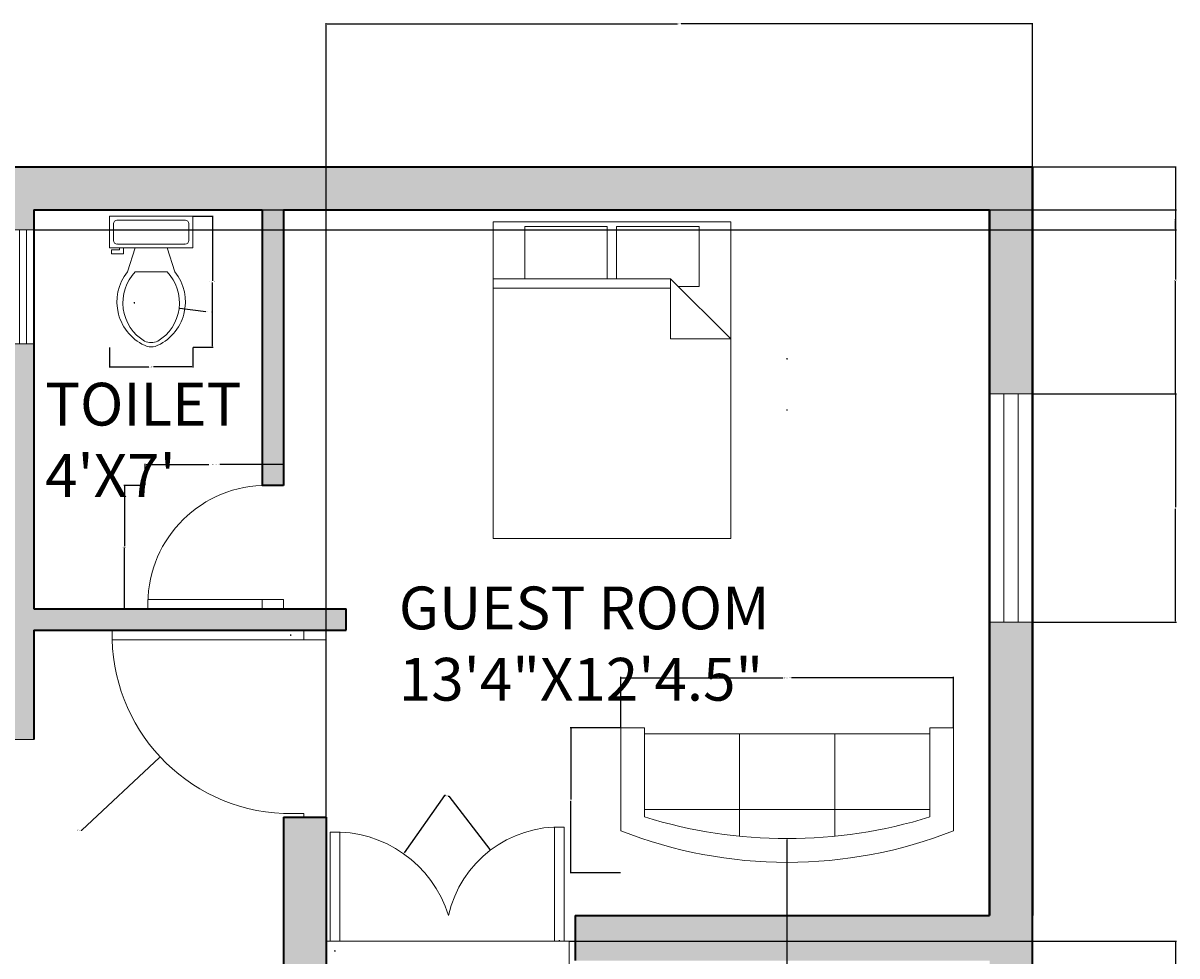
# Model space of a CAD drawing. Units: feet. Extents: x 1699 to 2359, y 1819 to 2211.
# Tile 4 of 4: x 2117 to 2359, y 2014 to 2211. Entities that reach past the tile are written whole.
import ezdxf

# ---------------------------------------------------------------- set-up
doc = ezdxf.new("R2010")
doc.units = ezdxf.units.FT
for name, color, linetype, lineweight in [('A-ANNO-DIMS', 2, 'Continuous', 18), ('A-AREA-IDEN', 7, 'Continuous', 18), ('A-DOOR', 4, 'Continuous', 18), ('A-FLOR', 7, 'Continuous', 18), ('A-FLOR-FIXT', 9, 'Continuous', 18), ('A-FURN', 8, 'Continuous', 18), ('A-GLAZ', 3, 'Continuous', 18), ('A-WALL', 7, 'Continuous', 35), ('A-WALL-PATT', 1, 'Continuous', 13)]:
    doc.layers.add(name, color=color, linetype=linetype, lineweight=lineweight)
doc.styles.get("Standard").update_dxf_attribs({"font": 'arial.ttf'})
doc.dimstyles.get("Standard").update_dxf_attribs({"dimtxt": 0.18, "dimasz": 0.18, "dimexe": 0.18, "dimexo": 0.0625, "dimgap": 0.09, "dimtad": 0, "dimtih": 1, "dimtoh": 1, "dimdec": 4, "dimzin": 0, "dimdsep": 46, "dimtxsty": 'Standard', "dimcen": 0.09, "dimadec": 0, "dimazin": 0, "dimtfac": 1, "dimtdec": 4, "dimtofl": 0, "dimtmove": 0, "dimatfit": 3, "dimfxl": 1, "dimtolj": 1, "dimtzin": 0, "dimarcsym": 0})

# ---------------------------------------------------------------- blocks, each defined once
blk = doc.blocks.new('Toilet - top')
for p, q in [((9.5, -6), (9.5, -2)), ((-10, -8.5), (-8, -8.5)), ((-10, -9.5), (-10, -8.5)), ((-8, -8.5), (-8, -8)), ((-7, -8), (-7, -9.5)), ((-4, -8), (-6, -14)), ((4, -8), (6, -14)), ((-7, -9.5), (-10, -9.5)), ((4, -14), (-4, -14))]:
    blk.add_line(p, q)
blk.add_lwpolyline([(10.5, -8), (10.5, 0), (-10.5, 0), (-10.5, -8)], close=True)
for points in [[(-9.5, -2), (-9.5, -6)], [(8.5, -1), (-8.5, -1)], [(-8.5, -7), (8.5, -7)]]:
    blk.add_lwpolyline(points)
for centre, radius, start, end in [((-8.62, -1.88), 0.884, 81.8699, 188.1301), ((8.62, -1.88), 0.884, 351.8699, 98.1301), ((-8.62, -6.12), 0.884, 171.8699, 278.1301), ((8.62, -6.12), 0.884, 261.8699, 8.1301), ((3.52, -21.58), 12.17, 141.4691, 247.9714), ((4.2, -21.82), 11.33, 136.3677, 238.9468), ((-3.52, -21.58), 12.17, 292.0284, 38.5307), ((-4.2, -21.82), 11.33, 301.053, 43.6321), ((0, -27.88), 4, 245.7318, 294.2682), ((0, -29), 4, 254.8605, 285.1395)]:
    blk.add_arc(centre, radius, start, end)
blk = doc.blocks.new('Bed - Queen')
for p, q in [((0, -80.00003), (0, 0)), ((0, 0), (59.99999, 0)), ((59.99999, 0), (59.99999, -80.00003)), ((7.99999, -1.2), (28.79998, -1.2)), ((7.99999, -14.4), (7.99999, -1.2)), ((28.79998, -1.2), (28.79998, -14.4)), ((31.19999, -1.2), (51.99999, -1.2)), ((31.19999, -14.4), (31.19999, -1.2)), ((51.99999, -1.2), (51.99999, -16.4)), ((0, -14.4), (44.8, -14.4)), ((59.99999, -29.6), (44.8, -14.4)), ((44.8, -14.4), (44.8, -29.6)), ((44.8, -16.8), (0, -16.8)), ((51.99999, -16.4), (46.79936, -16.4)), ((44.8, -29.6), (59.99999, -29.6)), ((59.99999, -80.00003), (0, -80.00003))]:
    blk.add_line(p, q)
blk = doc.blocks.new('Sofa - Roundback 7 ft.')
for p, q in [((-12.00002, -32.4421), (-12.00003, -6.5971)), ((11.99997, -32.4421), (11.99998, -6.5971)), ((-36.000027, -34), (-36.000027, -11.4696)), ((35.99998, -34), (35.99998, -11.4696)), ((-35.999844, -13.3819), (35.9998, -13.3819)), ((-36.000027, -32.4421), (35.99998, -32.4421))]:
    blk.add_line(p, q)
for points in [[(-36.000027, -34), (-42.000027, -34), (-42.000027, -8)], [(41.99998, -8), (41.99998, -34), (35.99998, -34)]]:
    blk.add_lwpolyline(points)
for centre, radius, start, end in [((0, -114.25), 114.25, 68.43141, 111.5686), ((-0.00001, -127.1968), 121.1968, 72.72033, 107.2797)]:
    blk.add_arc(centre, radius, start, end)
blk = doc.blocks.new('WIN-24-PARTITION')
for p, q in [((0, 24), (4.5, 24)), ((0, 0), (0, 24)), ((1.5, 0), (1.5, 24)), ((3, 0), (3, 24)), ((4.5, 24), (4.5, 0)), ((4.5, 0), (0, 0))]:
    blk.add_line(p, q)
blk = doc.blocks.new('DOOR-SWING-24')
for p, q in [((0.02, 0), (0.02, 2)), ((0.02, 2), (28.52, 2)), ((24.02, 0), (0.02, 0))]:
    blk.add_line(p, q)
blk.add_arc((25.02, 1), 25.02, 92.2906, 182.2906)
blk = doc.blocks.new('*D12')
at = {"layer": 'A-ANNO-DIMS', "color": 0, "lineweight": -2, "transparency": 16777216}
for p, q in [((2242.38, 2062.41), (2242.38, 2073.03)), ((2242.56, 2072.85), (2276.47, 2072.85)), ((2312.2, 2072.85), (2278.28, 2072.85)), ((2312.38, 2062.41), (2312.38, 2073.03))]:
    blk.add_line(p, q, dxfattribs=at)
at = {"layer": 'A-ANNO-DIMS', "color": 0, "transparency": 16777216}
for points in [[(2242.56, 2072.88), (2242.56, 2072.82), (2242.38, 2072.85)], [(2312.2, 2072.88), (2312.2, 2072.82), (2312.38, 2072.85)]]:
    blk.add_solid(points, dxfattribs=at)
at = {"layer": 'Defpoints', "color": 0, "transparency": 16777216}
for p in [(2242.38, 2072.85), (2242.38, 2062.35), (2312.38, 2062.35)]:
    blk.add_point(p, dxfattribs=at)
at = {"layer": 'A-ANNO-DIMS', "color": 0, "transparency": 16777216, "insert": (2277.38, 2072.85), "char_height": 0.18, "attachment_point": 5}
blk.add_mtext('\\A1;SOFA 70 TYP.', dxfattribs=at)
blk = doc.blocks.new('*D13')
at = {"layer": 'A-ANNO-DIMS', "color": 0, "lineweight": -2, "transparency": 16777216}
for p, q in [((2242.31, 2062.35), (2231.7, 2062.35)), ((2231.88, 2062.17), (2231.88, 2047.25)), ((2231.88, 2031.97), (2231.88, 2046.89)), ((2242.31, 2031.79), (2231.7, 2031.79))]:
    blk.add_line(p, q, dxfattribs=at)
at = {"layer": 'A-ANNO-DIMS', "color": 0, "transparency": 16777216}
for points in [[(2231.85, 2062.17), (2231.91, 2062.17), (2231.88, 2062.35)], [(2231.85, 2031.97), (2231.91, 2031.97), (2231.88, 2031.79)]]:
    blk.add_solid(points, dxfattribs=at)
at = {"layer": 'Defpoints', "color": 0, "transparency": 16777216}
for p in [(2242.38, 2062.35), (2231.88, 2031.79), (2242.38, 2031.79)]:
    blk.add_point(p, dxfattribs=at)
at = {"layer": 'A-ANNO-DIMS', "color": 0, "transparency": 16777216, "insert": (2231.88, 2047.07), "char_height": 0.18, "attachment_point": 5}
blk.add_mtext('\\A1;31 TYP.', dxfattribs=at)
blk = doc.blocks.new('*D14')
at = {"layer": 'A-ANNO-DIMS', "color": 0, "lineweight": -2, "transparency": 16777216}
for p, q in [((2152.43, 2169.97), (2156.68, 2169.97)), ((2156.5, 2169.79), (2156.5, 2156.38)), ((2156.5, 2142.61), (2156.5, 2156.02)), ((2152.43, 2142.43), (2156.68, 2142.43))]:
    blk.add_line(p, q, dxfattribs=at)
at = {"layer": 'A-ANNO-DIMS', "color": 0, "transparency": 16777216}
for points in [[(2156.47, 2169.79), (2156.53, 2169.79), (2156.5, 2169.97)], [(2156.47, 2142.61), (2156.53, 2142.61), (2156.5, 2142.43)]]:
    blk.add_solid(points, dxfattribs=at)
at = {"layer": 'Defpoints', "color": 0, "transparency": 16777216}
for p in [(2152.37, 2169.97), (2156.5, 2169.97), (2152.37, 2142.43)]:
    blk.add_point(p, dxfattribs=at)
at = {"layer": 'A-ANNO-DIMS', "color": 0, "transparency": 16777216, "insert": (2156.5, 2156.2), "char_height": 0.18, "attachment_point": 5}
blk.add_mtext('\\A1;WC 28 TYP.', dxfattribs=at)
blk = doc.blocks.new('*D15')
at = {"layer": 'A-ANNO-DIMS', "color": 0, "lineweight": -2, "transparency": 16777216}
for p, q in [((2134.87, 2142.37), (2134.87, 2138.12)), ((2152.37, 2142.37), (2152.37, 2138.12)), ((2135.05, 2138.3), (2143.1, 2138.3)), ((2152.19, 2138.3), (2144.13, 2138.3))]:
    blk.add_line(p, q, dxfattribs=at)
at = {"layer": 'A-ANNO-DIMS', "color": 0, "transparency": 16777216}
for points in [[(2135.05, 2138.33), (2135.05, 2138.27), (2134.87, 2138.3)], [(2152.19, 2138.33), (2152.19, 2138.27), (2152.37, 2138.3)]]:
    blk.add_solid(points, dxfattribs=at)
at = {"layer": 'Defpoints', "color": 0, "transparency": 16777216}
for p in [(2134.87, 2142.43), (2152.37, 2142.43), (2152.37, 2138.3)]:
    blk.add_point(p, dxfattribs=at)
at = {"layer": 'A-ANNO-DIMS', "color": 0, "transparency": 16777216, "insert": (2143.62, 2138.3), "char_height": 0.18, "attachment_point": 5}
blk.add_mtext('\\A1;18 TYP.', dxfattribs=at)
blk = doc.blocks.new('*D18')
at = {"layer": 'A-ANNO-DIMS', "color": 0, "lineweight": -2, "transparency": 16777216}
for p, q in [((2142.37, 2113.41), (2142.37, 2117.89)), ((2142.55, 2117.71), (2155.77, 2117.71)), ((2171.25, 2117.71), (2158.03, 2117.71)), ((2171.43, 2113.41), (2171.43, 2117.89))]:
    blk.add_line(p, q, dxfattribs=at)
at = {"layer": 'A-ANNO-DIMS', "color": 0, "transparency": 16777216}
for points in [[(2142.55, 2117.74), (2142.55, 2117.68), (2142.37, 2117.71)], [(2171.25, 2117.74), (2171.25, 2117.68), (2171.43, 2117.71)]]:
    blk.add_solid(points, dxfattribs=at)
at = {"layer": 'Defpoints', "color": 0, "transparency": 16777216}
for p in [(2171.43, 2117.71), (2142.37, 2113.35), (2171.43, 2113.35)]:
    blk.add_point(p, dxfattribs=at)
at = {"layer": 'A-ANNO-DIMS', "color": 0, "transparency": 16777216, "insert": (2156.9, 2117.71), "char_height": 0.18, "attachment_point": 5}
blk.add_mtext('\\A1;DOOR D1 29 TYP.', dxfattribs=at)
blk = doc.blocks.new('*D19')
at = {"layer": 'A-ANNO-DIMS', "color": 0, "lineweight": -2, "transparency": 16777216}
for p, q in [((2142.31, 2113.35), (2137.84, 2113.35)), ((2138.02, 2113.17), (2138.02, 2100.53)), ((2138.02, 2087.53), (2138.02, 2100.17)), ((2142.31, 2087.35), (2137.84, 2087.35))]:
    blk.add_line(p, q, dxfattribs=at)
at = {"layer": 'A-ANNO-DIMS', "color": 0, "transparency": 16777216}
for points in [[(2137.99, 2113.17), (2138.05, 2113.17), (2138.02, 2113.35)], [(2137.99, 2087.53), (2138.05, 2087.53), (2138.02, 2087.35)]]:
    blk.add_solid(points, dxfattribs=at)
at = {"layer": 'Defpoints', "color": 0, "transparency": 16777216}
for p in [(2138.02, 2113.35), (2142.37, 2113.35), (2142.37, 2087.35)]:
    blk.add_point(p, dxfattribs=at)
at = {"layer": 'A-ANNO-DIMS', "color": 0, "transparency": 16777216, "insert": (2138.02, 2100.35), "char_height": 0.18, "attachment_point": 5}
blk.add_mtext('\\A1;26 TYP.', dxfattribs=at)
blk = doc.blocks.new('*D22')
at = {"layer": 'A-ANNO-DIMS', "color": 0, "lineweight": -2, "transparency": 16777216}
for p, q in [((2180.43, 1853.41), (2180.43, 2210.63)), ((2328.93, 1848.91), (2328.93, 2210.63)), ((2180.61, 2210.45), (2254.29, 2210.45)), ((2328.75, 2210.45), (2255.06, 2210.45))]:
    blk.add_line(p, q, dxfattribs=at)
at = {"layer": 'A-ANNO-DIMS', "color": 0, "transparency": 16777216}
for points in [[(2180.61, 2210.48), (2180.61, 2210.42), (2180.43, 2210.45)], [(2328.75, 2210.48), (2328.75, 2210.42), (2328.93, 2210.45)]]:
    blk.add_solid(points, dxfattribs=at)
at = {"layer": 'Defpoints', "color": 0, "transparency": 16777216}
for p in [(2328.93, 2210.45), (2180.43, 1853.35), (2328.93, 1848.85)]:
    blk.add_point(p, dxfattribs=at)
at = {"layer": 'A-ANNO-DIMS', "color": 0, "transparency": 16777216, "insert": (2254.68, 2210.45), "char_height": 0.18, "attachment_point": 5}
blk.add_mtext('\\A1;148.5', dxfattribs=at)
blk = doc.blocks.new('*D35')
at = {"layer": 'A-ANNO-DIMS', "color": 0, "lineweight": -2, "transparency": 16777216}
for p, q in [((2231.55, 2017.45), (2359.21, 2017.45)), ((2359.03, 2017.27), (2359.03, 1976.45)), ((2359.03, 1935.26), (2359.03, 1976.08)), ((2231.55, 1935.08), (2359.21, 1935.08))]:
    blk.add_line(p, q, dxfattribs=at)
at = {"layer": 'A-ANNO-DIMS', "color": 0, "transparency": 16777216}
for points in [[(2359, 2017.27), (2359.06, 2017.27), (2359.03, 2017.45)], [(2359, 1935.26), (2359.06, 1935.26), (2359.03, 1935.08)]]:
    blk.add_solid(points, dxfattribs=at)
at = {"layer": 'Defpoints', "color": 0, "transparency": 16777216}
for p in [(2231.49, 2017.45), (2359.03, 2017.45), (2231.49, 1935.08)]:
    blk.add_point(p, dxfattribs=at)
at = {"layer": 'A-ANNO-DIMS', "color": 0, "transparency": 16777216, "insert": (2359.03, 1976.26), "char_height": 0.18, "attachment_point": 5}
blk.add_mtext('\\A1;82.37', dxfattribs=at)
blk = doc.blocks.new('*D36')
at = {"layer": 'A-ANNO-DIMS', "color": 0, "lineweight": -2, "transparency": 16777216}
for p, q in [((2328.99, 2132.58), (2359.21, 2132.58)), ((2359.03, 2132.4), (2359.03, 2108.76)), ((2359.03, 2084.76), (2359.03, 2108.4)), ((2328.99, 2084.58), (2359.21, 2084.58))]:
    blk.add_line(p, q, dxfattribs=at)
at = {"layer": 'A-ANNO-DIMS', "color": 0, "transparency": 16777216}
for points in [[(2359, 2132.4), (2359.06, 2132.4), (2359.03, 2132.58)], [(2359, 2084.76), (2359.06, 2084.76), (2359.03, 2084.58)]]:
    blk.add_solid(points, dxfattribs=at)
at = {"layer": 'Defpoints', "color": 0, "transparency": 16777216}
for p in [(2328.93, 2132.58), (2359.03, 2132.58), (2328.93, 2084.58)]:
    blk.add_point(p, dxfattribs=at)
at = {"layer": 'A-ANNO-DIMS', "color": 0, "transparency": 16777216, "insert": (2359.03, 2108.58), "char_height": 0.18, "attachment_point": 5}
blk.add_mtext('\\A1;48', dxfattribs=at)
blk = doc.blocks.new('*D37')
at = {"layer": 'A-ANNO-DIMS', "color": 0, "lineweight": -2, "transparency": 16777216}
for p, q in [((2328.989154, 2180.349391), (2359.206654, 2180.349391)), ((2359.026654, 2180.169391), (2359.026654, 2156.643959)), ((2359.026654, 2132.758527), (2359.026654, 2156.283959)), ((2328.989154, 2132.578527), (2359.206654, 2132.578527))]:
    blk.add_line(p, q, dxfattribs=at)
at = {"layer": 'A-ANNO-DIMS', "color": 0, "transparency": 16777216}
for points in [[(2358.996654, 2180.169391), (2359.056654, 2180.169391), (2359.026654, 2180.349391)], [(2358.996654, 2132.758527), (2359.056654, 2132.758527), (2359.026654, 2132.578527)]]:
    blk.add_solid(points, dxfattribs=at)
at = {"layer": 'Defpoints', "color": 0, "transparency": 16777216}
for p in [(2328.926654, 2180.349391), (2359.026654, 2180.349391), (2328.926654, 2132.578527)]:
    blk.add_point(p, dxfattribs=at)
at = {"layer": 'A-ANNO-DIMS', "color": 0, "transparency": 16777216, "insert": (2359.026654, 2156.463959), "char_height": 0.18, "attachment_point": 5}
blk.add_mtext('\\A1;47.77', dxfattribs=at)
blk = doc.blocks.new('*D51')
at = {"layer": 'A-ANNO-DIMS', "color": 0, "lineweight": -2, "transparency": 16777216}
for p, q in [((2118.99, 2171.35), (2359.21, 2171.35)), ((2359.03, 2171.17), (2359.03, 2169.43)), ((2118.99, 2167.14), (2359.21, 2167.14)), ((2359.03, 2167.32), (2359.03, 2169.06))]:
    blk.add_line(p, q, dxfattribs=at)
at = {"layer": 'A-ANNO-DIMS', "color": 0, "transparency": 16777216}
for points in [[(2359, 2171.17), (2359.06, 2171.17), (2359.03, 2171.35)], [(2359, 2167.32), (2359.06, 2167.32), (2359.03, 2167.14)]]:
    blk.add_solid(points, dxfattribs=at)
at = {"layer": 'Defpoints', "color": 0, "transparency": 16777216}
for p in [(2118.93, 2171.35), (2118.93, 2167.14), (2359.03, 2167.14)]:
    blk.add_point(p, dxfattribs=at)
at = {"layer": 'A-ANNO-DIMS', "color": 0, "transparency": 16777216, "insert": (2359.03, 2169.25), "char_height": 0.18, "attachment_point": 5}
blk.add_mtext('\\A1;4.21', dxfattribs=at)
blk = doc.blocks.new('*D55')
at = {"layer": 'A-ANNO-DIMS', "color": 0, "lineweight": -2, "transparency": 16777216}
for p, q in [((2172.91, 2081.85), (2173.09, 2081.85)), ((2173, 2081.76), (2173, 2081.94)), ((2129.04, 2040.8), (2145.4, 2056.07)), ((2128.86, 2040.8), (2129.04, 2040.8))]:
    blk.add_line(p, q, dxfattribs=at)
at = {"layer": 'A-ANNO-DIMS', "color": 0, "transparency": 16777216}
blk.add_solid([(2145.38, 2056.1), (2145.42, 2056.05), (2145.53, 2056.2)], dxfattribs=at)
at = {"layer": 'Defpoints', "color": 0, "transparency": 16777216}
for p in [(2173, 2081.85), (2145.53, 2056.2)]:
    blk.add_point(p, dxfattribs=at)
at = {"layer": 'A-ANNO-DIMS', "color": 0, "transparency": 16777216, "insert": (2128.38, 2040.8), "char_height": 0.18, "attachment_point": 5}
blk.add_mtext('\\A1;R37.59', dxfattribs=at)
blk = doc.blocks.new('*D57')
at = {"layer": 'A-ANNO-DIMS', "color": 0, "lineweight": -2, "transparency": 16777216}
for p, q in [((2205.33, 2048.11), (2196.79, 2035.99)), ((2205.51, 2048.11), (2205.33, 2048.11)), ((2182.18, 2015.4), (2182.36, 2015.4)), ((2182.27, 2015.31), (2182.27, 2015.49))]:
    blk.add_line(p, q, dxfattribs=at)
at = {"layer": 'A-ANNO-DIMS', "color": 0, "transparency": 16777216}
blk.add_solid([(2196.76, 2036), (2196.81, 2035.97), (2196.68, 2035.84)], dxfattribs=at)
at = {"layer": 'Defpoints', "color": 0, "transparency": 16777216}
for p in [(2196.68, 2035.84), (2182.27, 2015.4)]:
    blk.add_point(p, dxfattribs=at)
at = {"layer": 'A-ANNO-DIMS', "color": 0, "transparency": 16777216, "insert": (2205.98, 2048.11), "char_height": 0.18, "attachment_point": 5}
blk.add_mtext('\\A1;R25.01', dxfattribs=at)
blk = doc.blocks.new('*D58')
at = {"layer": 'A-ANNO-DIMS', "color": 0, "lineweight": -2, "transparency": 16777216}
for p, q in [((2206.04, 2047.94), (2206.22, 2047.94)), ((2206.22, 2047.94), (2214.82, 2036.7)), ((2229.37, 2017.57), (2229.55, 2017.57)), ((2229.46, 2017.48), (2229.46, 2017.66))]:
    blk.add_line(p, q, dxfattribs=at)
at = {"layer": 'A-ANNO-DIMS', "color": 0, "transparency": 16777216}
blk.add_solid([(2214.85, 2036.71), (2214.8, 2036.68), (2214.93, 2036.55)], dxfattribs=at)
at = {"layer": 'Defpoints', "color": 0, "transparency": 16777216}
for p in [(2214.93, 2036.55), (2229.46, 2017.57)]:
    blk.add_point(p, dxfattribs=at)
at = {"layer": 'A-ANNO-DIMS', "color": 0, "transparency": 16777216, "insert": (2205.49, 2047.94), "char_height": 0.18, "attachment_point": 5}
blk.add_mtext('\\A1;R23.903', dxfattribs=at)
blk = doc.blocks.new('*D59')
at = {"layer": 'A-ANNO-DIMS', "color": 0, "lineweight": -2, "transparency": 16777216}
for p, q in [((2277.29, 2140.01), (2277.47, 2140.01)), ((2277.38, 2139.92), (2277.38, 2140.1)), ((2277.38, 1978.42), (2277.38, 2038.84)), ((2277.56, 1978.42), (2277.38, 1978.42))]:
    blk.add_line(p, q, dxfattribs=at)
at = {"layer": 'A-ANNO-DIMS', "color": 0, "transparency": 16777216}
blk.add_solid([(2277.41, 2038.84), (2277.35, 2038.84), (2277.38, 2039.02)], dxfattribs=at)
at = {"layer": 'Defpoints', "color": 0, "transparency": 16777216}
for p in [(2277.38, 2140.01), (2277.38, 2039.02)]:
    blk.add_point(p, dxfattribs=at)
at = {"layer": 'A-ANNO-DIMS', "color": 0, "transparency": 16777216, "insert": (2278.11, 1978.42), "char_height": 0.18, "attachment_point": 5}
blk.add_mtext('\\A1;2X R101', dxfattribs=at)
blk = doc.blocks.new('*D60')
at = {"layer": 'A-ANNO-DIMS', "color": 0, "lineweight": -2, "transparency": 16777216}
for p, q in [((2277.29, 2129.22), (2277.47, 2129.22)), ((2277.38, 2129.13), (2277.38, 2129.31)), ((2277.38, 1976.89), (2277.38, 2033.84)), ((2277.56, 1976.89), (2277.38, 1976.89))]:
    blk.add_line(p, q, dxfattribs=at)
at = {"layer": 'A-ANNO-DIMS', "color": 0, "transparency": 16777216}
blk.add_solid([(2277.41, 2033.84), (2277.35, 2033.84), (2277.38, 2034.02)], dxfattribs=at)
at = {"layer": 'Defpoints', "color": 0, "transparency": 16777216}
for p in [(2277.38, 2129.22), (2277.38, 2034.02)]:
    blk.add_point(p, dxfattribs=at)
at = {"layer": 'A-ANNO-DIMS', "color": 0, "transparency": 16777216, "insert": (2278.16, 1976.89), "char_height": 0.18, "attachment_point": 5}
blk.add_mtext('\\A1;2X R95.2', dxfattribs=at)
blk = doc.blocks.new('*D64')
at = {"layer": 'A-ANNO-DIMS', "color": 0, "lineweight": -2, "transparency": 16777216}
for p, q in [((2140.03, 2151.79), (2140.21, 2151.79)), ((2140.12, 2151.7), (2140.12, 2151.88)), ((2155.09, 2149.84), (2149.66, 2150.54))]:
    blk.add_line(p, q, dxfattribs=at)
at = {"layer": 'A-ANNO-DIMS', "color": 0, "transparency": 16777216}
blk.add_solid([(2149.66, 2150.57), (2149.65, 2150.52), (2149.48, 2150.57)], dxfattribs=at)
at = {"layer": 'Defpoints', "color": 0, "transparency": 16777216}
for p in [(2140.12, 2151.79), (2149.48, 2150.57)]:
    blk.add_point(p, dxfattribs=at)
at = {"layer": 'A-ANNO-DIMS', "color": 0, "transparency": 16777216, "insert": (2155.75, 2149.84), "char_height": 0.18, "attachment_point": 5}
blk.add_mtext('\\A1;4X R9.441', dxfattribs=at)

msp = doc.modelspace()

# ---------------------------------------------------------------- hatches: boundary and pattern name
at = {"layer": 'A-WALL-PATT'}
h = msp.add_hatch(color=256, dxfattribs=at)
h.dxf.hatch_style = 1
h.paths.add_polyline_path([(2180.4267, 1853.3494), (2180.4267, 1857.8494), (1955.4267, 1857.8494), (1955.4267, 1935.0782), (1991.4267, 1935.0782), (1991.4267, 1939.5782), (1955.4267, 1939.5782), (1955.4267, 2022.8494), (1950.9267, 2022.8494), (1950.9267, 1857.8494), (1784.4267, 1857.8494), (1784.4267, 1908.7829), (1775.4267, 1908.7829), (1775.4267, 1853.3494), (1733.9267, 1853.3494), (1733.9267, 2018.3494), (1775.4267, 2018.3494), (1775.4267, 2022.8494), (1738.4267, 2022.8494), (1738.4267, 2171.3494), (1898.4267, 2171.3494), (1898.4267, 2060.8494), (1902.9267, 2060.8494), (1902.9267, 2064.8494), (1955.4267, 2064.8494), (1955.4267, 2069.3494), (1902.9267, 2069.3494), (1902.9267, 2171.3494), (1950.9267, 2171.3494), (1950.9267, 2169.0373), (1955.4267, 2169.0373), (1955.4267, 2175.8494), (2114.4267, 2175.8494), (2114.4267, 2167.1408), (2118.9267, 2167.1408), (2118.9267, 2171.3494), (2166.9267, 2171.3494), (2166.9267, 2113.3494), (2171.4267, 2113.3494), (2171.4267, 2171.3494), (2319.9267, 2171.3494), (2319.9267, 2132.5785), (2328.9267, 2132.5785), (2328.9267, 2180.3494), (2309.4267, 2180.3494), (1729.4267, 2180.3494), (1729.4267, 1848.8494), (2180.4267, 1848.8494)])
h.paths.add_polyline_path([(1784.4267, 1987.6139), (1775.4267, 1987.6139), (1775.4267, 1944.7829), (1784.4267, 1944.7829)], flags=17)
h.paths.add_polyline_path([(1912.9267, 2022.8494), (1775.4267, 2022.8494), (1775.4267, 2013.6139), (1784.4267, 2013.6139), (1784.4267, 2018.3494), (1912.9267, 2018.3494)], flags=17)
h.paths.add_polyline_path([(2018.4267, 2135.3494), (2047.4307, 2135.3494), (2047.4307, 2139.8494), (1981.4267, 2139.8494), (1981.4267, 2135.3494), (2013.9267, 2135.3494), (2013.9267, 2059.8494), (2018.4267, 2059.8494)], flags=17)
h.paths.add_polyline_path([(2114.4267, 2139.8494), (2071.4307, 2139.8494), (2071.4307, 2135.3494), (2114.4267, 2135.3494)], flags=17)
h.paths.add_polyline_path([(2118.9267, 2143.1408), (2114.4267, 2143.1408), (2114.4267, 2059.8494), (2118.9267, 2059.8494), (2118.9267, 2082.8494), (2184.631, 2082.8494), (2184.631, 2087.3494), (2118.9267, 2087.3494)], flags=17)
h.paths.add_polyline_path([(2328.9267, 2084.5785), (2319.9267, 2084.5785), (2319.9267, 2022.8494), (2232.7955, 2022.8494), (2232.7955, 2013.3494), (2319.9267, 2013.3494), (2319.9267, 1998.3723), (2328.9267, 1998.3723)], flags=17)
h.paths.add_polyline_path([(2180.4267, 2043.5261), (2171.4267, 2043.5261), (2171.4267, 2006.4114), (2180.4267, 2006.4114)], flags=17)
h.paths.add_polyline_path([(2015.0526, 1939.5782), (1991.4267, 1939.5782), (1991.4267, 1935.0782), (2015.0526, 1935.0782)], flags=17)
h.paths.add_polyline_path([(2180.4267, 1939.5782), (2087.0526, 1939.5782), (2087.0526, 1935.0782), (2180.4267, 1935.0782)], flags=17)
h.paths.add_polyline_path([(2328.9267, 1868.1839), (2319.9267, 1868.1839), (2319.9267, 1853.3494), (2180.4267, 1853.3494), (2180.4267, 1848.8494), (2328.9267, 1848.8494)], flags=17)

# ---------------------------------------------------------------- linework, layer by layer
at = {"layer": 'A-DOOR'}
for p, q in [((2166.9267, 2089.3494), (2166.9267, 2087.3494)), ((2171.4267, 2089.3494), (2171.4267, 2087.3494)), ((2171.4267, 2082.8494), (2135.4267, 2082.8494)), ((2135.4267, 2082.8494), (2135.4267, 2080.8494)), ((2175.7191, 2082.7861), (2175.7191, 2080.8494)), ((2180.4267, 2082.8494), (2180.4267, 2080.8494)), ((2135.4267, 2080.8494), (2180.4267, 2080.8494)), ((2175.7191, 2044.2932), (2171.4267, 2044.2932)), ((2175.7191, 2044.2932), (2175.7191, 2043.5261)), ((2230.4592, 2041.4514), (2228.4592, 2041.4514)), ((2228.4592, 2041.4514), (2228.4592, 2017.4514)), ((2230.4592, 2017.4514), (2230.4592, 2041.4514)), ((2181.2703, 2022.8494), (2181.2703, 2040.3914)), ((2181.2703, 2040.3914), (2183.2703, 2040.3914)), ((2183.2703, 2040.3914), (2183.2703, 2017.4514)), ((2181.2703, 2022.8494), (2181.2703, 2017.4514)), ((2180.4267, 2017.4514), (2182.4016, 2017.4514)), ((2228.4592, 2017.4514), (2180.4267, 2017.4514)), ((2182.4592, 2017.4514), (2183.2703, 2017.4514)), ((2228.4592, 2017.4514), (2230.4592, 2017.4514)), ((2230.4592, 2017.4514), (2232.7955, 2017.4514))]:
    msp.add_line(p, q, dxfattribs=at)
for centre, radius, start, end in [((2173.0026, 2081.8494), 37.5892, 178.475559, 267.597193), ((2229.4592, 2017.5698), 23.9025, 87.602239, 167.239361), ((2182.2703, 2015.3995), 25.012, 17.328754, 92.291346)]:
    msp.add_arc(centre, radius, start, end, dxfattribs=at)
at = {"layer": 'A-FLOR'}
for p, q in [((2013.9267, 2059.8494), (2118.9267, 2059.8494)), ((2231.4915, 1935.0782), (2231.4915, 2017.4514))]:
    msp.add_line(p, q, dxfattribs=at)
at = {"layer": 'A-GLAZ'}
for p, q in [((2328.9267, 2132.5785), (2319.9267, 2132.5785)), ((2319.9267, 2132.5785), (2319.9267, 2084.5785)), ((2322.9267, 2132.5785), (2322.9267, 2084.5785)), ((2325.9267, 2132.5785), (2325.9267, 2084.5785)), ((2328.9267, 2084.5785), (2328.9267, 2132.5785)), ((2319.9267, 2084.5785), (2328.9267, 2084.5785))]:
    msp.add_line(p, q, dxfattribs=at)
at = {"layer": 'A-WALL'}
for p, q in [((1729.4267, 2180.3494), (2309.4267, 2180.3494)), ((2309.4267, 2180.3494), (2328.9267, 2180.3494)), ((2328.9267, 2180.3494), (2328.9267, 2022.8494)), ((2328.9267, 1998.3723), (2328.9267, 2180.2967)), ((2118.9267, 2171.3494), (2118.9267, 2087.3494)), ((2118.9267, 2171.3494), (2166.9267, 2171.3494)), ((2166.9267, 2171.3494), (2166.9267, 2113.3494)), ((2171.4267, 2171.3494), (2171.4267, 2113.3494)), ((2171.4267, 2171.3494), (2319.9267, 2171.3494)), ((2319.9267, 2171.3494), (2319.9267, 2022.8494)), ((2319.9267, 2022.8494), (2319.9267, 2171.3494)), ((2171.4267, 2113.3494), (2166.9267, 2113.3494)), ((2118.9267, 2087.3494), (2184.631, 2087.3494)), ((2184.631, 2082.8494), (2184.631, 2087.3494)), ((2118.9267, 2082.8494), (2184.631, 2082.8494)), ((2118.9267, 2082.8494), (2118.9267, 2059.8494)), ((2171.4267, 2043.5261), (2180.4267, 2043.5261)), ((2171.4267, 2043.5261), (2171.4267, 2006.4114)), ((2180.4267, 2043.5261), (2180.4267, 2006.4114)), ((2232.7955, 2022.8494), (2319.9267, 2022.8494)), ((2232.7955, 2022.8494), (2232.7955, 2013.3494))]:
    msp.add_line(p, q, dxfattribs=at)

# ---------------------------------------------------------------- block references
at = {"layer": 'A-DOOR'}
msp.add_blockref('DOOR-SWING-24', (2142.908, 2087.349), dxfattribs=at)
at = {"layer": 'A-FLOR-FIXT', "xscale": 0.8333333333333331, "yscale": 0.8333333333333331, "zscale": 0.8333333333333331}
msp.add_blockref('Toilet - top', (2143.6153, 2169.9691), dxfattribs=at)
at = {"layer": 'A-FURN', "xscale": 0.8333333333333331, "yscale": 0.8333333333333331, "zscale": 0.8333333333333331}
msp.add_blockref('Bed - Queen', (2215.5092, 2168.8318), dxfattribs=at)
at = {"layer": 'A-FURN', "xscale": 0.8333333333333331, "yscale": 0.8333333333333331, "zscale": 0.8333333333333331, "rotation": 180}
msp.add_blockref('Sofa - Roundback 7 ft.', (2277.3765, 2034.0163), dxfattribs=at)
at = {"layer": 'A-GLAZ', "rotation": 180}
msp.add_blockref('WIN-24-PARTITION', (2118.9263, 2167.1411), dxfattribs=at)

# ---------------------------------------------------------------- texts
at = {"layer": 'A-AREA-IDEN', "char_height": 9, "attachment_point": 1}
for s, width, insert in [("{\\fCambria|b0|i0|c0|p18;TOILET\\P4'X7'}", 39.448387, (2121.305, 2134.933)), ('{\\fCambria|b0|i0|c0|p18;GUEST ROOM\\P13\'4"X12\'4.5"}', 85.168581, (2195.7031, 2092.0543))]:
    msp.add_mtext_dynamic_manual_height_columns(s, width=width, gutter_width=12.5, heights=[0], dxfattribs=dict(at, insert=insert))

# ---------------------------------------------------------------- dimensions: what is measured, and where the dimension line sits
at = {"layer": 'A-ANNO-DIMS'}
dim = msp.add_linear_dim(base=(2328.9267, 2210.4494), p1=(2180.4267, 1853.3494), p2=(2328.9267, 1848.8494), dimstyle='Standard', override={"dimdec": 1, "dimlfac": 1, "dimrnd": 0, "dimzin": 0, "dimdsep": 46, "dimlunit": 2}, dxfattribs=at)
dim.commit()
dim.dimension.update_dxf_attribs({"geometry": '*D22', "text_midpoint": (2254.6767, 2210.4494)})
for base, p1, p2, override, picture, middle in [((2359.0267, 2180.3494), (2328.9267, 2132.5785), (2328.9267, 2180.3494), {"dimdec": 2, "dimlfac": 1, "dimrnd": 0, "dimzin": 0, "dimdsep": 46, "dimlunit": 2}, '*D37', (2359.0267, 2156.464)), ((2359.0267, 2167.1408), (2118.9267, 2171.3494), (2118.9267, 2167.1408), {"dimdec": 2, "dimlfac": 1, "dimrnd": 0, "dimzin": 0, "dimdsep": 46, "dimlunit": 2}, '*D51', (2359.0267, 2169.2451)), ((2359.0267, 2132.5785), (2328.9267, 2084.5785), (2328.9267, 2132.5785), {"dimdec": 0, "dimlfac": 1, "dimrnd": 0, "dimzin": 0, "dimdsep": 46, "dimlunit": 2}, '*D36', (2359.0267, 2108.5785)), ((2359.0267, 2017.4514), (2231.4915, 1935.0782), (2231.4915, 2017.4514), {"dimdec": 2, "dimlfac": 1, "dimrnd": 0, "dimzin": 0, "dimdsep": 46, "dimlunit": 2}, '*D35', (2359.0267, 1976.2648))]:
    dim = msp.add_linear_dim(base=base, p1=p1, p2=p2, angle=90, dimstyle='Standard', override=override, dxfattribs=at)
    dim.commit()
    dim.dimension.update_dxf_attribs({"geometry": picture, "text_midpoint": middle})
for base, p1, p2, angle, text, picture, middle in [((2156.4961, 2169.9691), (2152.3653, 2142.4305), (2152.3653, 2169.9691), 90, 'WC <> TYP.', '*D14', (2156.4961, 2156.1998)), ((2138.0165, 2113.3494), (2142.3744, 2087.3494), (2142.3744, 2113.3494), 90, '<> TYP.', '*D19', (2138.0165, 2100.3494)), ((2242.3765, 2072.8497), (2312.3765, 2062.3497), (2242.3765, 2062.3497), 180, 'SOFA <> TYP.', '*D12', (2277.3765, 2072.8497)), ((2231.8765, 2031.7941), (2242.3765, 2062.3497), (2242.3765, 2031.7941), 270, '<> TYP.', '*D13', (2231.8765, 2047.0719))]:
    dim = msp.add_linear_dim(base=base, p1=p1, p2=p2, angle=angle, text=text, dimstyle='Standard', override={"dimdec": 0, "dimlfac": 1, "dimrnd": 0, "dimzin": 0, "dimdsep": 46, "dimlunit": 2}, dxfattribs=at)
    dim.commit()
    dim.dimension.update_dxf_attribs({"geometry": picture, "text_midpoint": middle})
for center, mpoint, text, override, picture, middle in [((2140.1154, 2151.7879), (2149.4773, 2150.5681), '4X <>', {"dimdec": 3, "dimlfac": 1, "dimrnd": 0, "dimzin": 0, "dimdsep": 46, "dimlunit": 2}, '*D64', (2155.0944, 2149.8362)), ((2277.3765, 2140.0137), (2277.377, 2039.0163), '2X <>', {"dimdec": 0, "dimlfac": 1, "dimrnd": 0, "dimzin": 0, "dimdsep": 46, "dimlunit": 2}, '*D59', (2278.1098, 1978.4179)), ((2277.3765, 2129.2247), (2277.377, 2034.0163), '2X <>', {"dimdec": 1, "dimlfac": 1, "dimrnd": 0, "dimzin": 0, "dimdsep": 46, "dimlunit": 2}, '*D60', (2278.1612, 1976.8913))]:
    dim = msp.add_radius_dim(center=center, mpoint=mpoint, text=text, dimstyle='Standard', override=override, dxfattribs=at)
    dim.commit()
    dim.dimension.update_dxf_attribs({"geometry": picture, "text_midpoint": middle, "dimtype": 164})
for base, p1, p2, text, picture, middle in [((2152.3653038443, 2138.2997496963), (2134.8653038443, 2142.4305302143), (2152.3653038443, 2142.4305302143), '<> TYP.', '*D15', (2143.6153038443, 2138.2997496963)), ((2171.4267, 2117.7072), (2142.3744, 2113.3494), (2171.4267, 2113.3494), 'DOOR D1 <> TYP.', '*D18', (2156.9005, 2117.7072))]:
    dim = msp.add_linear_dim(base=base, p1=p1, p2=p2, text=text, dimstyle='Standard', override={"dimdec": 0, "dimlfac": 1, "dimrnd": 0, "dimzin": 0, "dimdsep": 46, "dimlunit": 2}, dxfattribs=at)
    dim.commit()
    dim.dimension.update_dxf_attribs({"geometry": picture, "text_midpoint": middle})
for center, mpoint, override, picture, middle in [((2173.0026, 2081.8494), (2145.528, 2056.196), {"dimdec": 2, "dimlfac": 1, "dimrnd": 0, "dimzin": 0, "dimdsep": 46, "dimlunit": 2}, '*D55', (2128.3832, 2040.804)), ((2182.2703, 2015.3995), (2196.6843, 2035.8405), {"dimdec": 2, "dimlfac": 1, "dimrnd": 0, "dimzin": 0, "dimdsep": 46, "dimlunit": 2}, '*D57', (2205.9752, 2048.1051)), ((2229.4592, 2017.5698), (2214.9341, 2036.5528), {"dimdec": 3, "dimlfac": 1, "dimrnd": 0, "dimzin": 0, "dimdsep": 46, "dimlunit": 2}, '*D58', (2205.4894, 2047.9426))]:
    dim = msp.add_radius_dim(center=center, mpoint=mpoint, dimstyle='Standard', override=override, dxfattribs=at)
    dim.commit()
    dim.dimension.update_dxf_attribs({"geometry": picture, "text_midpoint": middle, "dimtype": 164})

doc.saveas('drawing.dxf')
